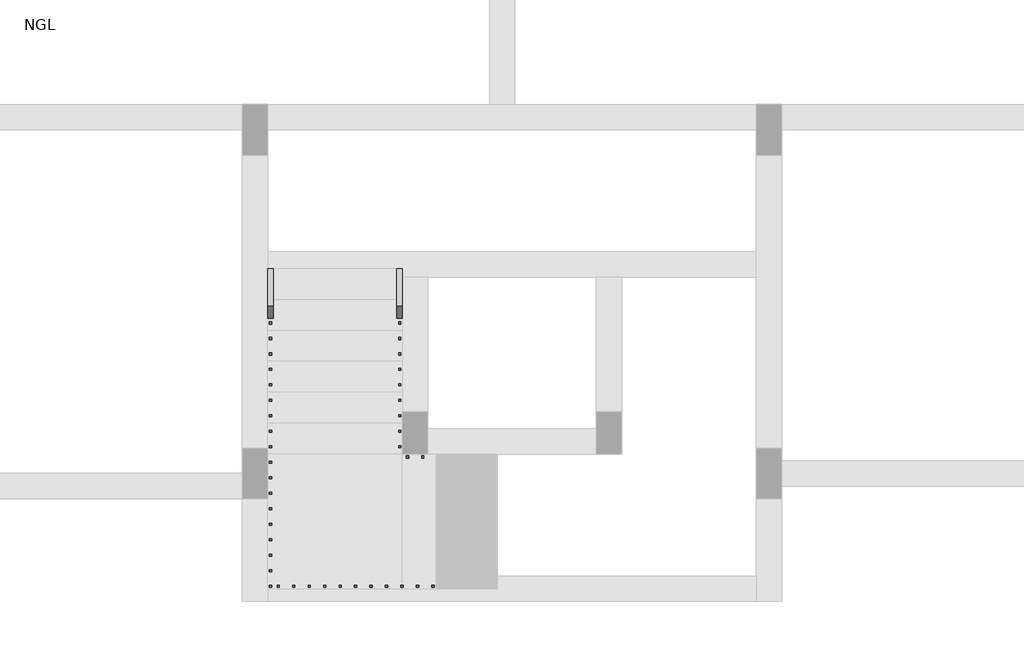
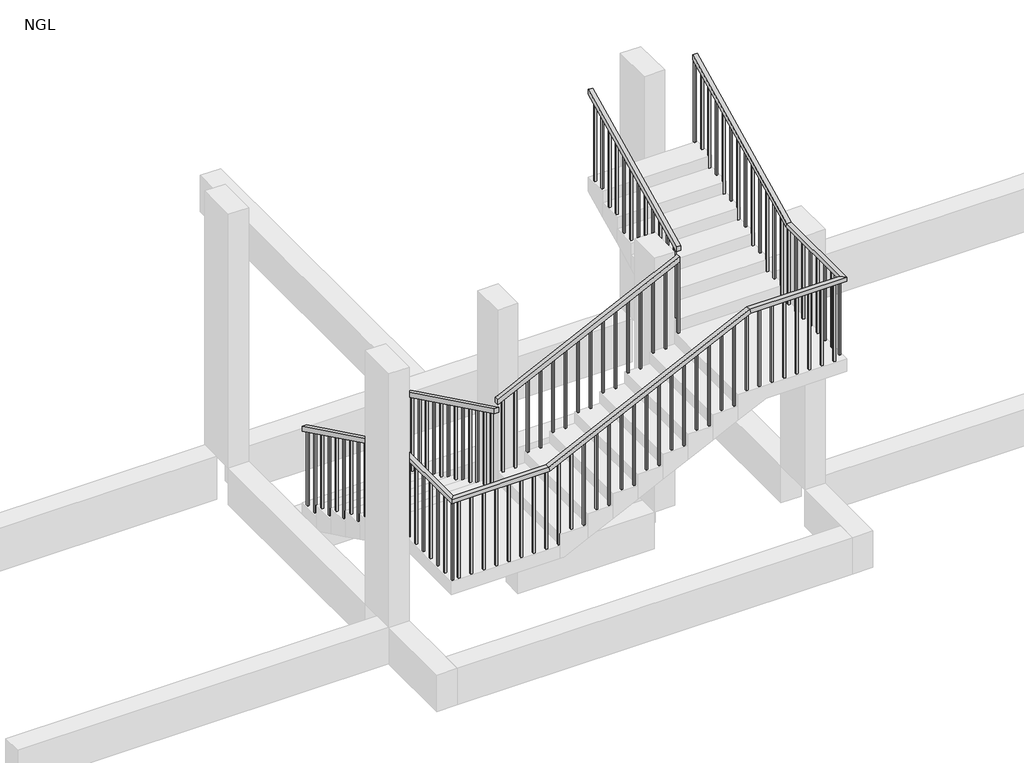
# One storey, part 2 of 2: 2 railings.
"""IFC4 building model written with IfcOpenShell, lengths in millimetres."""

from ifc_helpers import new_model, si_unit, frame, origin, place, context, project, spatial, polyline, outline, extrude, faceted_brep, element, save

model = new_model("IFC4")

# Units and contexts
model_context = context("Model", 3, world=origin())
ifc_project = project(units=[si_unit("LENGTHUNIT", "METRE", prefix="MILLI")], contexts=[model_context])

# Site, building, storey
site = spatial("IfcSite", under=ifc_project)
building = spatial("IfcBuilding", under=site)
storey = spatial("IfcBuildingStorey", under=building, Name="NGL", Elevation=0.0)

# Railings
placement = place(None, origin())
element("IfcRailing", 1, ObjectType="900mm", at=placement, inside=storey, context=model_context, shape_type="SolidModel", body=[
    faceted_brep([(5667245.0165246, -3595922.4258983, 1036.3636364), (5667245.0165246, -3595922.4258983, 980.7263867), (5667195.0165246, -3595922.4258983, 980.7263867), (5667195.0165246, -3595922.4258983, 1036.3636364), (5667245.0165246, -3597746.1784624, 1926.4621742), (5667245.0165246, -3597757.7288111, 1876.4621742), (5667195.0165246, -3597757.7288111, 1876.4621742), (5667195.0165246, -3597746.1784624, 1926.4621742), (5667245.0165246, -3598767.6258983, 1876.4621742), (5667245.0165246, -3598767.6258983, 1926.4621742), (5668280.0541869, -3598767.6258983, 1926.4621742), (5668291.4712079, -3598767.6258983, 1876.4621742), (5667195.0165246, -3598817.6258983, 1876.4621742), (5668291.4712079, -3598817.6258983, 1876.4621742), (5667195.0165246, -3598817.6258983, 1926.4621742), (5668280.0541869, -3598817.6258983, 1926.4621742), (5671563.8165246, -3598767.6258983, 2959.9014622), (5671563.8165246, -3598767.6258983, 3009.9014622), (5671563.8165246, -3597746.1784624, 3009.9014622), (5671563.8165246, -3597734.6281137, 2959.9014622), (5671613.8165246, -3598817.6258983, 2959.9014622), (5671613.8165246, -3597734.6281137, 2959.9014622), (5671613.8165246, -3598817.6258983, 3009.9014622), (5671613.8165246, -3597746.1784624, 3009.9014622), (5670528.7788622, -3598767.6258983, 3009.9014622), (5670540.1958832, -3598767.6258983, 2959.9014622), (5670540.1958832, -3598817.6258983, 2959.9014622), (5670528.7788622, -3598817.6258983, 3009.9014622), (5671563.8165246, -3595922.4258983, 3900.0), (5671613.8165246, -3595922.4258983, 3900.0), (5671613.8165246, -3595922.4258983, 3844.3627504), (5671563.8165246, -3595922.4258983, 3844.3627504)], [[[0, 1, 2, 3]], [[1, 0, 4, 5]], [[2, 1, 5, 6]], [[3, 2, 6, 7]], [[0, 3, 7, 4]], [[8, 9, 10, 11]], [[12, 8, 11, 13]], [[14, 12, 13, 15]], [[9, 14, 15, 10]], [[16, 17, 18, 19]], [[20, 16, 19, 21]], [[22, 20, 21, 23]], [[17, 22, 23, 18]], [[5, 4, 9, 8]], [[6, 5, 8, 12]], [[7, 6, 12, 14]], [[4, 7, 14, 9]], [[11, 10, 24, 25]], [[13, 11, 25, 26]], [[15, 13, 26, 27]], [[10, 15, 27, 24]], [[25, 24, 17, 16]], [[26, 25, 16, 20]], [[27, 26, 20, 22]], [[24, 27, 22, 17]], [[28, 29, 30, 31]], [[19, 18, 28, 31]], [[21, 19, 31, 30]], [[23, 21, 30, 29]], [[18, 23, 29, 28]]]),
    extrude(outline(polyline([(-3595932.6258983, 2863.6363636), (-3595932.6258983, 3839.3845503), (-3595912.6258983, 3849.1457269), (-3595912.6258983, 2863.6363636), (-3595932.6258983, 2863.6363636)])), frame((5671578.8165246, 0.0, 0.0), z_axis=(1.0, 0.0, 0.0), x_axis=(0.0, 1.0, 0.0)), (0.0, 0.0, 1.0), 20.0),
    extrude(outline(polyline([(-3596072.6258983, 2863.6363636), (-3596072.6258983, 3771.0563145), (-3596052.6258983, 3780.817491), (-3596052.6258983, 2863.6363636), (-3596072.6258983, 2863.6363636)])), frame((5671578.8165246, 0.0, 0.0), z_axis=(1.0, 0.0, 0.0), x_axis=(0.0, 1.0, 0.0)), (0.0, 0.0, 1.0), 20.0),
    extrude(outline(polyline([(-3596212.6258983, 2727.2727273), (-3596212.6258983, 3702.7280787), (-3596192.6258983, 3712.4892552), (-3596192.6258983, 2727.2727273), (-3596212.6258983, 2727.2727273)])), frame((5671578.8165246, 0.0, 0.0), z_axis=(1.0, 0.0, 0.0), x_axis=(0.0, 1.0, 0.0)), (0.0, 0.0, 1.0), 20.0),
    extrude(outline(polyline([(-3596352.6258983, 2727.2727273), (-3596352.6258983, 3634.3998428), (-3596332.6258983, 3644.1610194), (-3596332.6258983, 2727.2727273), (-3596352.6258983, 2727.2727273)])), frame((5671578.8165246, 0.0, 0.0), z_axis=(1.0, 0.0, 0.0), x_axis=(0.0, 1.0, 0.0)), (0.0, 0.0, 1.0), 20.0),
    extrude(outline(polyline([(-3596492.6258983, 2590.9090909), (-3596492.6258983, 3566.071607), (-3596472.6258983, 3575.8327835), (-3596472.6258983, 2590.9090909), (-3596492.6258983, 2590.9090909)])), frame((5671578.8165246, 0.0, 0.0), z_axis=(1.0, 0.0, 0.0), x_axis=(0.0, 1.0, 0.0)), (0.0, 0.0, 1.0), 20.0),
    extrude(outline(polyline([(-3596632.6258983, 2590.9090909), (-3596632.6258983, 3497.7433712), (-3596612.6258983, 3507.5045477), (-3596612.6258983, 2590.9090909), (-3596632.6258983, 2590.9090909)])), frame((5671578.8165246, 0.0, 0.0), z_axis=(1.0, 0.0, 0.0), x_axis=(0.0, 1.0, 0.0)), (0.0, 0.0, 1.0), 20.0),
    extrude(outline(polyline([(-3596772.6258983, 2454.5454545), (-3596772.6258983, 3429.4151353), (-3596752.6258983, 3439.1763119), (-3596752.6258983, 2454.5454545), (-3596772.6258983, 2454.5454545)])), frame((5671578.8165246, 0.0, 0.0), z_axis=(1.0, 0.0, 0.0), x_axis=(0.0, 1.0, 0.0)), (0.0, 0.0, 1.0), 20.0),
    extrude(outline(polyline([(-3596912.6258983, 2454.5454545), (-3596912.6258983, 3361.0868995), (-3596892.6258983, 3370.8480761), (-3596892.6258983, 2454.5454545), (-3596912.6258983, 2454.5454545)])), frame((5671578.8165246, 0.0, 0.0), z_axis=(1.0, 0.0, 0.0), x_axis=(0.0, 1.0, 0.0)), (0.0, 0.0, 1.0), 20.0),
    extrude(outline(polyline([(-3597052.6258983, 2318.1818182), (-3597052.6258983, 3292.7586637), (-3597032.6258983, 3302.5198402), (-3597032.6258983, 2318.1818182), (-3597052.6258983, 2318.1818182)])), frame((5671578.8165246, 0.0, 0.0), z_axis=(1.0, 0.0, 0.0), x_axis=(0.0, 1.0, 0.0)), (0.0, 0.0, 1.0), 20.0),
    extrude(outline(polyline([(-3597192.6258983, 2318.1818182), (-3597192.6258983, 3224.4304279), (-3597172.6258983, 3234.1916044), (-3597172.6258983, 2318.1818182), (-3597192.6258983, 2318.1818182)])), frame((5671578.8165246, 0.0, 0.0), z_axis=(1.0, 0.0, 0.0), x_axis=(0.0, 1.0, 0.0)), (0.0, 0.0, 1.0), 20.0),
    extrude(outline(polyline([(-3597332.6258983, 2181.8181818), (-3597332.6258983, 3156.0322155), (-3597312.6258983, 3165.6682488), (-3597312.6258983, 2181.8181818), (-3597332.6258983, 2181.8181818)])), frame((5671578.8165246, 0.0, 0.0), z_axis=(1.0, 0.0, 0.0), x_axis=(0.0, 1.0, 0.0)), (0.0, 0.0, 1.0), 20.0),
    extrude(outline(polyline([(-3597472.6258983, 2181.8181818), (-3597472.6258983, 3087.7739562), (-3597452.6258983, 3097.5351327), (-3597452.6258983, 2181.8181818), (-3597472.6258983, 2181.8181818)])), frame((5671578.8165246, 0.0, 0.0), z_axis=(1.0, 0.0, 0.0), x_axis=(0.0, 1.0, 0.0)), (0.0, 0.0, 1.0), 20.0),
    extrude(outline(polyline([(-3597612.6258983, 2045.4545455), (-3597612.6258983, 3019.4457204), (-3597592.6258983, 3029.2068969), (-3597592.6258983, 2045.4545455), (-3597612.6258983, 2045.4545455)])), frame((5671578.8165246, 0.0, 0.0), z_axis=(1.0, 0.0, 0.0), x_axis=(0.0, 1.0, 0.0)), (0.0, 0.0, 1.0), 20.0),
    extrude(outline(polyline([(-3597752.6258983, 2045.4545455), (-3597752.6258983, 2951.1174845), (-3597732.6258983, 2960.8786611), (-3597732.6258983, 2045.4545455), (-3597752.6258983, 2045.4545455)])), frame((5671578.8165246, 0.0, 0.0), z_axis=(1.0, 0.0, 0.0), x_axis=(0.0, 1.0, 0.0)), (0.0, 0.0, 1.0), 20.0),
    extrude(outline(polyline([(5671598.8165246, -3597892.6258983), (5671578.8165246, -3597892.6258983), (5671578.8165246, -3597872.6258983), (5671598.8165246, -3597872.6258983), (5671598.8165246, -3597892.6258983)])), frame((0.0, 0.0, 2045.4545455), z_axis=(0.0, 0.0, 1.0), x_axis=(1.0, 0.0, 0.0)), (0.0, 0.0, 1.0), 914.4469167),
    extrude(outline(polyline([(5671598.8165246, -3598032.6258983), (5671578.8165246, -3598032.6258983), (5671578.8165246, -3598012.6258983), (5671598.8165246, -3598012.6258983), (5671598.8165246, -3598032.6258983)])), frame((0.0, 0.0, 2045.4545455), z_axis=(0.0, 0.0, 1.0), x_axis=(1.0, 0.0, 0.0)), (0.0, 0.0, 1.0), 914.4469167),
    extrude(outline(polyline([(5671598.8165246, -3598172.6258983), (5671578.8165246, -3598172.6258983), (5671578.8165246, -3598152.6258983), (5671598.8165246, -3598152.6258983), (5671598.8165246, -3598172.6258983)])), frame((0.0, 0.0, 2045.4545455), z_axis=(0.0, 0.0, 1.0), x_axis=(1.0, 0.0, 0.0)), (0.0, 0.0, 1.0), 914.4469167),
    extrude(outline(polyline([(5671598.8165246, -3598312.6258983), (5671578.8165246, -3598312.6258983), (5671578.8165246, -3598292.6258983), (5671598.8165246, -3598292.6258983), (5671598.8165246, -3598312.6258983)])), frame((0.0, 0.0, 2045.4545455), z_axis=(0.0, 0.0, 1.0), x_axis=(1.0, 0.0, 0.0)), (0.0, 0.0, 1.0), 914.4469167),
    extrude(outline(polyline([(5671598.8165246, -3598452.6258983), (5671578.8165246, -3598452.6258983), (5671578.8165246, -3598432.6258983), (5671598.8165246, -3598432.6258983), (5671598.8165246, -3598452.6258983)])), frame((0.0, 0.0, 2045.4545455), z_axis=(0.0, 0.0, 1.0), x_axis=(1.0, 0.0, 0.0)), (0.0, 0.0, 1.0), 914.4469167),
    extrude(outline(polyline([(5671598.8165246, -3598592.6258983), (5671578.8165246, -3598592.6258983), (5671578.8165246, -3598572.6258983), (5671598.8165246, -3598572.6258983), (5671598.8165246, -3598592.6258983)])), frame((0.0, 0.0, 2045.4545455), z_axis=(0.0, 0.0, 1.0), x_axis=(1.0, 0.0, 0.0)), (0.0, 0.0, 1.0), 914.4469167),
    extrude(outline(polyline([(5671598.8165246, -3598732.6258983), (5671578.8165246, -3598732.6258983), (5671578.8165246, -3598712.6258983), (5671598.8165246, -3598712.6258983), (5671598.8165246, -3598732.6258983)])), frame((0.0, 0.0, 2045.4545455), z_axis=(0.0, 0.0, 1.0), x_axis=(1.0, 0.0, 0.0)), (0.0, 0.0, 1.0), 914.4469167),
    extrude(outline(polyline([(5671480.0165246, -3598802.6258983), (5671480.0165246, -3598782.6258983), (5671500.0165246, -3598782.6258983), (5671500.0165246, -3598802.6258983), (5671480.0165246, -3598802.6258983)])), frame((0.0, 0.0, 2045.4545455), z_axis=(0.0, 0.0, 1.0), x_axis=(1.0, 0.0, 0.0)), (0.0, 0.0, 1.0), 914.4469167),
    extrude(outline(polyline([(5671340.0165246, -3598802.6258983), (5671340.0165246, -3598782.6258983), (5671360.0165246, -3598782.6258983), (5671360.0165246, -3598802.6258983), (5671340.0165246, -3598802.6258983)])), frame((0.0, 0.0, 2045.4545455), z_axis=(0.0, 0.0, 1.0), x_axis=(1.0, 0.0, 0.0)), (0.0, 0.0, 1.0), 914.4469167),
    extrude(outline(polyline([(5671200.0165246, -3598802.6258983), (5671200.0165246, -3598782.6258983), (5671220.0165246, -3598782.6258983), (5671220.0165246, -3598802.6258983), (5671200.0165246, -3598802.6258983)])), frame((0.0, 0.0, 2045.4545455), z_axis=(0.0, 0.0, 1.0), x_axis=(1.0, 0.0, 0.0)), (0.0, 0.0, 1.0), 914.4469167),
    extrude(outline(polyline([(5671060.0165246, -3598802.6258983), (5671060.0165246, -3598782.6258983), (5671080.0165246, -3598782.6258983), (5671080.0165246, -3598802.6258983), (5671060.0165246, -3598802.6258983)])), frame((0.0, 0.0, 2045.4545455), z_axis=(0.0, 0.0, 1.0), x_axis=(1.0, 0.0, 0.0)), (0.0, 0.0, 1.0), 914.4469167),
    extrude(outline(polyline([(5670920.0165246, -3598802.6258983), (5670920.0165246, -3598782.6258983), (5670940.0165246, -3598782.6258983), (5670940.0165246, -3598802.6258983), (5670920.0165246, -3598802.6258983)])), frame((0.0, 0.0, 2045.4545455), z_axis=(0.0, 0.0, 1.0), x_axis=(1.0, 0.0, 0.0)), (0.0, 0.0, 1.0), 914.4469167),
    extrude(outline(polyline([(5670780.0165246, -3598802.6258983), (5670780.0165246, -3598782.6258983), (5670800.0165246, -3598782.6258983), (5670800.0165246, -3598802.6258983), (5670780.0165246, -3598802.6258983)])), frame((0.0, 0.0, 2045.4545455), z_axis=(0.0, 0.0, 1.0), x_axis=(1.0, 0.0, 0.0)), (0.0, 0.0, 1.0), 914.4469167),
    extrude(outline(polyline([(5670640.0165246, -3598802.6258983), (5670640.0165246, -3598782.6258983), (5670660.0165246, -3598782.6258983), (5670660.0165246, -3598802.6258983), (5670640.0165246, -3598802.6258983)])), frame((0.0, 0.0, 2045.4545455), z_axis=(0.0, 0.0, 1.0), x_axis=(1.0, 0.0, 0.0)), (0.0, 0.0, 1.0), 914.4469167),
    extrude(outline(polyline([(2940.5429804, 5670500.0165246), (2045.4545455, 5670500.0165246), (2045.4545455, 5670520.0165246), (2950.1790136, 5670520.0165246), (2940.5429804, 5670500.0165246)])), frame((0.0, -3598802.6258983, 0.0), z_axis=(0.0, 1.0, 0.0), x_axis=(0.0, 0.0, 1.0)), (0.0, 0.0, 1.0), 20.0),
    extrude(outline(polyline([(2873.0907476, 5670360.0165246), (1909.0909091, 5670360.0165246), (1909.0909091, 5670380.0165246), (2882.7267808, 5670380.0165246), (2873.0907476, 5670360.0165246)])), frame((0.0, -3598802.6258983, 0.0), z_axis=(0.0, 1.0, 0.0), x_axis=(0.0, 0.0, 1.0)), (0.0, 0.0, 1.0), 20.0),
    extrude(outline(polyline([(2805.6385148, 5670220.0165246), (1909.0909091, 5670220.0165246), (1909.0909091, 5670240.0165246), (2815.274548, 5670240.0165246), (2805.6385148, 5670220.0165246)])), frame((0.0, -3598802.6258983, 0.0), z_axis=(0.0, 1.0, 0.0), x_axis=(0.0, 0.0, 1.0)), (0.0, 0.0, 1.0), 20.0),
    extrude(outline(polyline([(2738.186282, 5670080.0165246), (1772.7272727, 5670080.0165246), (1772.7272727, 5670100.0165246), (2747.8223152, 5670100.0165246), (2738.186282, 5670080.0165246)])), frame((0.0, -3598802.6258983, 0.0), z_axis=(0.0, 1.0, 0.0), x_axis=(0.0, 0.0, 1.0)), (0.0, 0.0, 1.0), 20.0),
    extrude(outline(polyline([(2670.7340492, 5669940.0165246), (1772.7272727, 5669940.0165246), (1772.7272727, 5669960.0165246), (2680.3700824, 5669960.0165246), (2670.7340492, 5669940.0165246)])), frame((0.0, -3598802.6258983, 0.0), z_axis=(0.0, 1.0, 0.0), x_axis=(0.0, 0.0, 1.0)), (0.0, 0.0, 1.0), 20.0),
    extrude(outline(polyline([(2603.2818163, 5669800.0165246), (1636.3636364, 5669800.0165246), (1636.3636364, 5669820.0165246), (2612.9178496, 5669820.0165246), (2603.2818163, 5669800.0165246)])), frame((0.0, -3598802.6258983, 0.0), z_axis=(0.0, 1.0, 0.0), x_axis=(0.0, 0.0, 1.0)), (0.0, 0.0, 1.0), 20.0),
    extrude(outline(polyline([(2535.8295835, 5669660.0165246), (1636.3636364, 5669660.0165246), (1636.3636364, 5669680.0165246), (2545.4656168, 5669680.0165246), (2535.8295835, 5669660.0165246)])), frame((0.0, -3598802.6258983, 0.0), z_axis=(0.0, 1.0, 0.0), x_axis=(0.0, 0.0, 1.0)), (0.0, 0.0, 1.0), 20.0),
    extrude(outline(polyline([(2468.3773507, 5669520.0165246), (1500.0, 5669520.0165246), (1500.0, 5669540.0165246), (2478.013384, 5669540.0165246), (2468.3773507, 5669520.0165246)])), frame((0.0, -3598802.6258983, 0.0), z_axis=(0.0, 1.0, 0.0), x_axis=(0.0, 0.0, 1.0)), (0.0, 0.0, 1.0), 20.0),
    extrude(outline(polyline([(2400.9251179, 5669380.0165246), (1500.0, 5669380.0165246), (1500.0, 5669400.0165246), (2410.5611512, 5669400.0165246), (2400.9251179, 5669380.0165246)])), frame((0.0, -3598802.6258983, 0.0), z_axis=(0.0, 1.0, 0.0), x_axis=(0.0, 0.0, 1.0)), (0.0, 0.0, 1.0), 20.0),
    extrude(outline(polyline([(2333.4728851, 5669240.0165246), (1363.6363636, 5669240.0165246), (1363.6363636, 5669260.0165246), (2343.1089184, 5669260.0165246), (2333.4728851, 5669240.0165246)])), frame((0.0, -3598802.6258983, 0.0), z_axis=(0.0, 1.0, 0.0), x_axis=(0.0, 0.0, 1.0)), (0.0, 0.0, 1.0), 20.0),
    extrude(outline(polyline([(2266.0206523, 5669100.0165246), (1363.6363636, 5669100.0165246), (1363.6363636, 5669120.0165246), (2275.6566856, 5669120.0165246), (2266.0206523, 5669100.0165246)])), frame((0.0, -3598802.6258983, 0.0), z_axis=(0.0, 1.0, 0.0), x_axis=(0.0, 0.0, 1.0)), (0.0, 0.0, 1.0), 20.0),
    extrude(outline(polyline([(2198.5684195, 5668960.0165246), (1227.2727273, 5668960.0165246), (1227.2727273, 5668980.0165246), (2208.2044528, 5668980.0165246), (2198.5684195, 5668960.0165246)])), frame((0.0, -3598802.6258983, 0.0), z_axis=(0.0, 1.0, 0.0), x_axis=(0.0, 0.0, 1.0)), (0.0, 0.0, 1.0), 20.0),
    extrude(outline(polyline([(2131.1161867, 5668820.0165246), (1227.2727273, 5668820.0165246), (1227.2727273, 5668840.0165246), (2140.75222, 5668840.0165246), (2131.1161867, 5668820.0165246)])), frame((0.0, -3598802.6258983, 0.0), z_axis=(0.0, 1.0, 0.0), x_axis=(0.0, 0.0, 1.0)), (0.0, 0.0, 1.0), 20.0),
    extrude(outline(polyline([(2063.6639539, 5668680.0165246), (1090.9090909, 5668680.0165246), (1090.9090909, 5668700.0165246), (2073.2999871, 5668700.0165246), (2063.6639539, 5668680.0165246)])), frame((0.0, -3598802.6258983, 0.0), z_axis=(0.0, 1.0, 0.0), x_axis=(0.0, 0.0, 1.0)), (0.0, 0.0, 1.0), 20.0),
    extrude(outline(polyline([(1996.2117211, 5668540.0165246), (1090.9090909, 5668540.0165246), (1090.9090909, 5668560.0165246), (2005.8477543, 5668560.0165246), (1996.2117211, 5668540.0165246)])), frame((0.0, -3598802.6258983, 0.0), z_axis=(0.0, 1.0, 0.0), x_axis=(0.0, 0.0, 1.0)), (0.0, 0.0, 1.0), 20.0),
    extrude(outline(polyline([(1928.7594883, 5668400.0165246), (954.5454545, 5668400.0165246), (954.5454545, 5668420.0165246), (1938.3955215, 5668420.0165246), (1928.7594883, 5668400.0165246)])), frame((0.0, -3598802.6258983, 0.0), z_axis=(0.0, 1.0, 0.0), x_axis=(0.0, 0.0, 1.0)), (0.0, 0.0, 1.0), 20.0),
    extrude(outline(polyline([(5668260.0165246, -3598802.6258983), (5668260.0165246, -3598782.6258983), (5668280.0165246, -3598782.6258983), (5668280.0165246, -3598802.6258983), (5668260.0165246, -3598802.6258983)])), frame((0.0, 0.0, 954.5454545), z_axis=(0.0, 0.0, 1.0), x_axis=(1.0, 0.0, 0.0)), (0.0, 0.0, 1.0), 921.9167196),
    extrude(outline(polyline([(5668120.0165246, -3598802.6258983), (5668120.0165246, -3598782.6258983), (5668140.0165246, -3598782.6258983), (5668140.0165246, -3598802.6258983), (5668120.0165246, -3598802.6258983)])), frame((0.0, 0.0, 954.5454545), z_axis=(0.0, 0.0, 1.0), x_axis=(1.0, 0.0, 0.0)), (0.0, 0.0, 1.0), 921.9167196),
    extrude(outline(polyline([(5667980.0165246, -3598802.6258983), (5667980.0165246, -3598782.6258983), (5668000.0165246, -3598782.6258983), (5668000.0165246, -3598802.6258983), (5667980.0165246, -3598802.6258983)])), frame((0.0, 0.0, 954.5454545), z_axis=(0.0, 0.0, 1.0), x_axis=(1.0, 0.0, 0.0)), (0.0, 0.0, 1.0), 921.9167196),
    extrude(outline(polyline([(5667840.0165246, -3598802.6258983), (5667840.0165246, -3598782.6258983), (5667860.0165246, -3598782.6258983), (5667860.0165246, -3598802.6258983), (5667840.0165246, -3598802.6258983)])), frame((0.0, 0.0, 954.5454545), z_axis=(0.0, 0.0, 1.0), x_axis=(1.0, 0.0, 0.0)), (0.0, 0.0, 1.0), 921.9167196),
    extrude(outline(polyline([(5667700.0165246, -3598802.6258983), (5667700.0165246, -3598782.6258983), (5667720.0165246, -3598782.6258983), (5667720.0165246, -3598802.6258983), (5667700.0165246, -3598802.6258983)])), frame((0.0, 0.0, 954.5454545), z_axis=(0.0, 0.0, 1.0), x_axis=(1.0, 0.0, 0.0)), (0.0, 0.0, 1.0), 921.9167196),
    extrude(outline(polyline([(5667560.0165246, -3598802.6258983), (5667560.0165246, -3598782.6258983), (5667580.0165246, -3598782.6258983), (5667580.0165246, -3598802.6258983), (5667560.0165246, -3598802.6258983)])), frame((0.0, 0.0, 954.5454545), z_axis=(0.0, 0.0, 1.0), x_axis=(1.0, 0.0, 0.0)), (0.0, 0.0, 1.0), 921.9167196),
    extrude(outline(polyline([(5667420.0165246, -3598802.6258983), (5667420.0165246, -3598782.6258983), (5667440.0165246, -3598782.6258983), (5667440.0165246, -3598802.6258983), (5667420.0165246, -3598802.6258983)])), frame((0.0, 0.0, 954.5454545), z_axis=(0.0, 0.0, 1.0), x_axis=(1.0, 0.0, 0.0)), (0.0, 0.0, 1.0), 921.9167196),
    extrude(outline(polyline([(5667280.0165246, -3598802.6258983), (5667280.0165246, -3598782.6258983), (5667300.0165246, -3598782.6258983), (5667300.0165246, -3598802.6258983), (5667280.0165246, -3598802.6258983)])), frame((0.0, 0.0, 954.5454545), z_axis=(0.0, 0.0, 1.0), x_axis=(1.0, 0.0, 0.0)), (0.0, 0.0, 1.0), 921.9167196),
    extrude(outline(polyline([(5667210.0165246, -3598782.4258983), (5667230.0165246, -3598782.4258983), (5667230.0165246, -3598802.4258983), (5667210.0165246, -3598802.4258983), (5667210.0165246, -3598782.4258983)])), frame((0.0, 0.0, 954.5454545), z_axis=(0.0, 0.0, 1.0), x_axis=(1.0, 0.0, 0.0)), (0.0, 0.0, 1.0), 921.9167196),
    extrude(outline(polyline([(5667210.0165246, -3598642.4258983), (5667230.0165246, -3598642.4258983), (5667230.0165246, -3598662.4258983), (5667210.0165246, -3598662.4258983), (5667210.0165246, -3598642.4258983)])), frame((0.0, 0.0, 954.5454545), z_axis=(0.0, 0.0, 1.0), x_axis=(1.0, 0.0, 0.0)), (0.0, 0.0, 1.0), 921.9167196),
    extrude(outline(polyline([(5667210.0165246, -3598502.4258983), (5667230.0165246, -3598502.4258983), (5667230.0165246, -3598522.4258983), (5667210.0165246, -3598522.4258983), (5667210.0165246, -3598502.4258983)])), frame((0.0, 0.0, 954.5454545), z_axis=(0.0, 0.0, 1.0), x_axis=(1.0, 0.0, 0.0)), (0.0, 0.0, 1.0), 921.9167196),
    extrude(outline(polyline([(5667210.0165246, -3598362.4258983), (5667230.0165246, -3598362.4258983), (5667230.0165246, -3598382.4258983), (5667210.0165246, -3598382.4258983), (5667210.0165246, -3598362.4258983)])), frame((0.0, 0.0, 954.5454545), z_axis=(0.0, 0.0, 1.0), x_axis=(1.0, 0.0, 0.0)), (0.0, 0.0, 1.0), 921.9167196),
    extrude(outline(polyline([(5667210.0165246, -3598222.4258983), (5667230.0165246, -3598222.4258983), (5667230.0165246, -3598242.4258983), (5667210.0165246, -3598242.4258983), (5667210.0165246, -3598222.4258983)])), frame((0.0, 0.0, 954.5454545), z_axis=(0.0, 0.0, 1.0), x_axis=(1.0, 0.0, 0.0)), (0.0, 0.0, 1.0), 921.9167196),
    extrude(outline(polyline([(5667210.0165246, -3598082.4258983), (5667230.0165246, -3598082.4258983), (5667230.0165246, -3598102.4258983), (5667210.0165246, -3598102.4258983), (5667210.0165246, -3598082.4258983)])), frame((0.0, 0.0, 954.5454545), z_axis=(0.0, 0.0, 1.0), x_axis=(1.0, 0.0, 0.0)), (0.0, 0.0, 1.0), 921.9167196),
    extrude(outline(polyline([(5667210.0165246, -3597942.4258983), (5667230.0165246, -3597942.4258983), (5667230.0165246, -3597962.4258983), (5667210.0165246, -3597962.4258983), (5667210.0165246, -3597942.4258983)])), frame((0.0, 0.0, 954.5454545), z_axis=(0.0, 0.0, 1.0), x_axis=(1.0, 0.0, 0.0)), (0.0, 0.0, 1.0), 921.9167196),
    extrude(outline(polyline([(5667210.0165246, -3597802.4258983), (5667230.0165246, -3597802.4258983), (5667230.0165246, -3597822.4258983), (5667210.0165246, -3597822.4258983), (5667210.0165246, -3597802.4258983)])), frame((0.0, 0.0, 954.5454545), z_axis=(0.0, 0.0, 1.0), x_axis=(1.0, 0.0, 0.0)), (0.0, 0.0, 1.0), 921.9167196),
    extrude(outline(polyline([(-3597662.4258983, 1829.9487463), (-3597662.4258983, 954.5454545), (-3597682.4258983, 954.5454545), (-3597682.4258983, 1839.7099229), (-3597662.4258983, 1829.9487463)])), frame((5667210.0165246, 0.0, 0.0), z_axis=(1.0, 0.0, 0.0), x_axis=(0.0, 1.0, 0.0)), (0.0, 0.0, 1.0), 20.0),
    extrude(outline(polyline([(-3597522.4258983, 1761.6205105), (-3597522.4258983, 818.1818182), (-3597542.4258983, 818.1818182), (-3597542.4258983, 1771.381687), (-3597522.4258983, 1761.6205105)])), frame((5667210.0165246, 0.0, 0.0), z_axis=(1.0, 0.0, 0.0), x_axis=(0.0, 1.0, 0.0)), (0.0, 0.0, 1.0), 20.0),
    extrude(outline(polyline([(-3597382.4258983, 1693.2922747), (-3597382.4258983, 818.1818182), (-3597402.4258983, 818.1818182), (-3597402.4258983, 1703.0534512), (-3597382.4258983, 1693.2922747)])), frame((5667210.0165246, 0.0, 0.0), z_axis=(1.0, 0.0, 0.0), x_axis=(0.0, 1.0, 0.0)), (0.0, 0.0, 1.0), 20.0),
    extrude(outline(polyline([(-3597242.4258983, 1624.9640388), (-3597242.4258983, 681.8181818), (-3597262.4258983, 681.8181818), (-3597262.4258983, 1634.7252154), (-3597242.4258983, 1624.9640388)])), frame((5667210.0165246, 0.0, 0.0), z_axis=(1.0, 0.0, 0.0), x_axis=(0.0, 1.0, 0.0)), (0.0, 0.0, 1.0), 20.0),
    extrude(outline(polyline([(-3597102.4258983, 1556.635803), (-3597102.4258983, 681.8181818), (-3597122.4258983, 681.8181818), (-3597122.4258983, 1566.3969796), (-3597102.4258983, 1556.635803)])), frame((5667210.0165246, 0.0, 0.0), z_axis=(1.0, 0.0, 0.0), x_axis=(0.0, 1.0, 0.0)), (0.0, 0.0, 1.0), 20.0),
    extrude(outline(polyline([(-3596962.4258983, 1488.3075672), (-3596962.4258983, 545.4545455), (-3596982.4258983, 545.4545455), (-3596982.4258983, 1498.0687437), (-3596962.4258983, 1488.3075672)])), frame((5667210.0165246, 0.0, 0.0), z_axis=(1.0, 0.0, 0.0), x_axis=(0.0, 1.0, 0.0)), (0.0, 0.0, 1.0), 20.0),
    extrude(outline(polyline([(-3596822.4258983, 1419.9793313), (-3596822.4258983, 545.4545455), (-3596842.4258983, 545.4545455), (-3596842.4258983, 1429.7405079), (-3596822.4258983, 1419.9793313)])), frame((5667210.0165246, 0.0, 0.0), z_axis=(1.0, 0.0, 0.0), x_axis=(0.0, 1.0, 0.0)), (0.0, 0.0, 1.0), 20.0),
    extrude(outline(polyline([(-3596682.4258983, 1351.6510955), (-3596682.4258983, 409.0909091), (-3596702.4258983, 409.0909091), (-3596702.4258983, 1361.4122721), (-3596682.4258983, 1351.6510955)])), frame((5667210.0165246, 0.0, 0.0), z_axis=(1.0, 0.0, 0.0), x_axis=(0.0, 1.0, 0.0)), (0.0, 0.0, 1.0), 20.0),
    extrude(outline(polyline([(-3596542.4258983, 1283.3228597), (-3596542.4258983, 409.0909091), (-3596562.4258983, 409.0909091), (-3596562.4258983, 1293.0840362), (-3596542.4258983, 1283.3228597)])), frame((5667210.0165246, 0.0, 0.0), z_axis=(1.0, 0.0, 0.0), x_axis=(0.0, 1.0, 0.0)), (0.0, 0.0, 1.0), 20.0),
    extrude(outline(polyline([(-3596402.4258983, 1214.9946239), (-3596402.4258983, 272.7272727), (-3596422.4258983, 272.7272727), (-3596422.4258983, 1224.7558004), (-3596402.4258983, 1214.9946239)])), frame((5667210.0165246, 0.0, 0.0), z_axis=(1.0, 0.0, 0.0), x_axis=(0.0, 1.0, 0.0)), (0.0, 0.0, 1.0), 20.0),
    extrude(outline(polyline([(-3596262.4258983, 1146.666388), (-3596262.4258983, 272.7272727), (-3596282.4258983, 272.7272727), (-3596282.4258983, 1156.4275646), (-3596262.4258983, 1146.666388)])), frame((5667210.0165246, 0.0, 0.0), z_axis=(1.0, 0.0, 0.0), x_axis=(0.0, 1.0, 0.0)), (0.0, 0.0, 1.0), 20.0),
    extrude(outline(polyline([(-3596122.4258983, 1078.3381522), (-3596122.4258983, 136.3636364), (-3596142.4258983, 136.3636364), (-3596142.4258983, 1088.0993287), (-3596122.4258983, 1078.3381522)])), frame((5667210.0165246, 0.0, 0.0), z_axis=(1.0, 0.0, 0.0), x_axis=(0.0, 1.0, 0.0)), (0.0, 0.0, 1.0), 20.0),
    extrude(outline(polyline([(-3595982.4258983, 1010.0099164), (-3595982.4258983, 136.3636364), (-3596002.4258983, 136.3636364), (-3596002.4258983, 1019.7710929), (-3595982.4258983, 1010.0099164)])), frame((5667210.0165246, 0.0, 0.0), z_axis=(1.0, 0.0, 0.0), x_axis=(0.0, 1.0, 0.0)), (0.0, 0.0, 1.0), 20.0),
])
element("IfcRailing", 2, ObjectType="900mm", at=placement, inside=storey, context=model_context, shape_type="SweptSolid", body=[
    extrude(outline(polyline([(-3595922.4258983, 1036.3636364), (-3595922.4258983, 980.7263867), (-3597624.2258983, 1811.3048991), (-3597624.2258983, 1866.9421488), (-3595922.4258983, 1036.3636364)])), frame((5668363.4165246, 0.0, 0.0), z_axis=(1.0, 0.0, 0.0), x_axis=(0.0, 1.0, 0.0)), (0.0, 0.0, 1.0), 50.0),
    extrude(outline(polyline([(1978.6713287, 5668388.4165246), (1923.170589, 5668388.4165246), (2902.191568, 5670420.4165245), (2957.6923077, 5670420.4165245), (1978.6713287, 5668388.4165246)])), frame((0.0, -3597649.2258983, 0.0), z_axis=(0.0, 1.0, 0.0), x_axis=(0.0, 0.0, 1.0)), (0.0, 0.0, 1.0), 50.0),
    extrude(outline(polyline([(-3597624.2258983, 3013.784238), (-3597624.2258983, 3069.4214876), (-3595922.4258983, 3900.0), (-3595922.4258983, 3844.3627504), (-3597624.2258983, 3013.784238)])), frame((5670395.4165245, 0.0, 0.0), z_axis=(1.0, 0.0, 0.0), x_axis=(0.0, 1.0, 0.0)), (0.0, 0.0, 1.0), 50.0),
    extrude(outline(polyline([(-3596024.2258983, 3794.6783617), (-3596004.2258983, 3804.4395383), (-3596004.2258983, 2863.6363636), (-3596024.2258983, 2863.6363636), (-3596024.2258983, 3794.6783617)])), frame((5670410.4165245, 0.0, 0.0), z_axis=(1.0, 0.0, 0.0), x_axis=(0.0, 1.0, 0.0)), (0.0, 0.0, 1.0), 20.0),
    extrude(outline(polyline([(-3596164.2258983, 3726.3501259), (-3596144.2258983, 3736.1113025), (-3596144.2258983, 2863.6363636), (-3596164.2258983, 2863.6363636), (-3596164.2258983, 3726.3501259)])), frame((5670410.4165245, 0.0, 0.0), z_axis=(1.0, 0.0, 0.0), x_axis=(0.0, 1.0, 0.0)), (0.0, 0.0, 1.0), 20.0),
    extrude(outline(polyline([(-3596304.2258983, 3658.0218901), (-3596284.2258983, 3667.7830666), (-3596284.2258983, 2727.2727273), (-3596304.2258983, 2727.2727273), (-3596304.2258983, 3658.0218901)])), frame((5670410.4165245, 0.0, 0.0), z_axis=(1.0, 0.0, 0.0), x_axis=(0.0, 1.0, 0.0)), (0.0, 0.0, 1.0), 20.0),
    extrude(outline(polyline([(-3596444.2258983, 3589.6936542), (-3596424.2258983, 3599.4548308), (-3596424.2258983, 2727.2727273), (-3596444.2258983, 2727.2727273), (-3596444.2258983, 3589.6936542)])), frame((5670410.4165245, 0.0, 0.0), z_axis=(1.0, 0.0, 0.0), x_axis=(0.0, 1.0, 0.0)), (0.0, 0.0, 1.0), 20.0),
    extrude(outline(polyline([(-3596584.2258983, 3521.3654184), (-3596564.2258983, 3531.126595), (-3596564.2258983, 2590.9090909), (-3596584.2258983, 2590.9090909), (-3596584.2258983, 3521.3654184)])), frame((5670410.4165245, 0.0, 0.0), z_axis=(1.0, 0.0, 0.0), x_axis=(0.0, 1.0, 0.0)), (0.0, 0.0, 1.0), 20.0),
    extrude(outline(polyline([(-3596724.2258983, 3453.0371826), (-3596704.2258983, 3462.7983591), (-3596704.2258983, 2590.9090909), (-3596724.2258983, 2590.9090909), (-3596724.2258983, 3453.0371826)])), frame((5670410.4165245, 0.0, 0.0), z_axis=(1.0, 0.0, 0.0), x_axis=(0.0, 1.0, 0.0)), (0.0, 0.0, 1.0), 20.0),
    extrude(outline(polyline([(-3596864.2258983, 3384.7089468), (-3596844.2258983, 3394.4701233), (-3596844.2258983, 2454.5454545), (-3596864.2258983, 2454.5454545), (-3596864.2258983, 3384.7089468)])), frame((5670410.4165245, 0.0, 0.0), z_axis=(1.0, 0.0, 0.0), x_axis=(0.0, 1.0, 0.0)), (0.0, 0.0, 1.0), 20.0),
    extrude(outline(polyline([(-3597004.2258983, 3316.3807109), (-3596984.2258983, 3326.1418875), (-3596984.2258983, 2454.5454545), (-3597004.2258983, 2454.5454545), (-3597004.2258983, 3316.3807109)])), frame((5670410.4165245, 0.0, 0.0), z_axis=(1.0, 0.0, 0.0), x_axis=(0.0, 1.0, 0.0)), (0.0, 0.0, 1.0), 20.0),
    extrude(outline(polyline([(-3597144.2258983, 3248.0524751), (-3597124.2258983, 3257.8136516), (-3597124.2258983, 2318.1818182), (-3597144.2258983, 2318.1818182), (-3597144.2258983, 3248.0524751)])), frame((5670410.4165245, 0.0, 0.0), z_axis=(1.0, 0.0, 0.0), x_axis=(0.0, 1.0, 0.0)), (0.0, 0.0, 1.0), 20.0),
    extrude(outline(polyline([(-3597284.2258983, 3179.7242393), (-3597264.2258983, 3189.4854158), (-3597264.2258983, 2318.1818182), (-3597284.2258983, 2318.1818182), (-3597284.2258983, 3179.7242393)])), frame((5670410.4165245, 0.0, 0.0), z_axis=(1.0, 0.0, 0.0), x_axis=(0.0, 1.0, 0.0)), (0.0, 0.0, 1.0), 20.0),
    extrude(outline(polyline([(-3597424.2258983, 3111.3960034), (-3597404.2258983, 3121.15718), (-3597404.2258983, 2181.8181818), (-3597424.2258983, 2181.8181818), (-3597424.2258983, 3111.3960034)])), frame((5670410.4165245, 0.0, 0.0), z_axis=(1.0, 0.0, 0.0), x_axis=(0.0, 1.0, 0.0)), (0.0, 0.0, 1.0), 20.0),
    extrude(outline(polyline([(-3597564.2258983, 3042.9877797), (-3597544.2258983, 3052.6238129), (-3597544.2258983, 2181.8181818), (-3597564.2258983, 2181.8181818), (-3597564.2258983, 3042.9877797)])), frame((5670410.4165245, 0.0, 0.0), z_axis=(1.0, 0.0, 0.0), x_axis=(0.0, 1.0, 0.0)), (0.0, 0.0, 1.0), 20.0),
    extrude(outline(polyline([(2045.4545455, 5670408.4165246), (2045.4545455, 5670428.4165246), (2906.0459813, 5670428.4165246), (2896.4099481, 5670408.4165246), (2045.4545455, 5670408.4165246)])), frame((0.0, -3597634.2258983, 0.0), z_axis=(0.0, 1.0, 0.0), x_axis=(0.0, 0.0, 1.0)), (0.0, 0.0, 1.0), 20.0),
    extrude(outline(polyline([(1909.0909091, 5670268.4165246), (1909.0909091, 5670288.4165246), (2838.5937485, 5670288.4165246), (2828.9577152, 5670268.4165246), (1909.0909091, 5670268.4165246)])), frame((0.0, -3597634.2258983, 0.0), z_axis=(0.0, 1.0, 0.0), x_axis=(0.0, 0.0, 1.0)), (0.0, 0.0, 1.0), 20.0),
    extrude(outline(polyline([(1909.0909091, 5670128.4165246), (1909.0909091, 5670148.4165246), (2771.1415157, 5670148.4165246), (2761.5054824, 5670128.4165246), (1909.0909091, 5670128.4165246)])), frame((0.0, -3597634.2258983, 0.0), z_axis=(0.0, 1.0, 0.0), x_axis=(0.0, 0.0, 1.0)), (0.0, 0.0, 1.0), 20.0),
    extrude(outline(polyline([(1772.7272727, 5669988.4165246), (1772.7272727, 5670008.4165246), (2703.6892829, 5670008.4165246), (2694.0532496, 5669988.4165246), (1772.7272727, 5669988.4165246)])), frame((0.0, -3597634.2258983, 0.0), z_axis=(0.0, 1.0, 0.0), x_axis=(0.0, 0.0, 1.0)), (0.0, 0.0, 1.0), 20.0),
    extrude(outline(polyline([(1772.7272727, 5669848.4165246), (1772.7272727, 5669868.4165246), (2636.2370501, 5669868.4165246), (2626.6010168, 5669848.4165246), (1772.7272727, 5669848.4165246)])), frame((0.0, -3597634.2258983, 0.0), z_axis=(0.0, 1.0, 0.0), x_axis=(0.0, 0.0, 1.0)), (0.0, 0.0, 1.0), 20.0),
    extrude(outline(polyline([(1636.3636364, 5669708.4165246), (1636.3636364, 5669728.4165246), (2568.7848173, 5669728.4165246), (2559.148784, 5669708.4165246), (1636.3636364, 5669708.4165246)])), frame((0.0, -3597634.2258983, 0.0), z_axis=(0.0, 1.0, 0.0), x_axis=(0.0, 0.0, 1.0)), (0.0, 0.0, 1.0), 20.0),
    extrude(outline(polyline([(1636.3636364, 5669568.4165246), (1636.3636364, 5669588.4165246), (2501.3325845, 5669588.4165246), (2491.6965512, 5669568.4165246), (1636.3636364, 5669568.4165246)])), frame((0.0, -3597634.2258983, 0.0), z_axis=(0.0, 1.0, 0.0), x_axis=(0.0, 0.0, 1.0)), (0.0, 0.0, 1.0), 20.0),
    extrude(outline(polyline([(1500.0, 5669428.4165246), (1500.0, 5669448.4165246), (2433.8803517, 5669448.4165246), (2424.2443184, 5669428.4165246), (1500.0, 5669428.4165246)])), frame((0.0, -3597634.2258983, 0.0), z_axis=(0.0, 1.0, 0.0), x_axis=(0.0, 0.0, 1.0)), (0.0, 0.0, 1.0), 20.0),
    extrude(outline(polyline([(1500.0, 5669288.4165246), (1500.0, 5669308.4165246), (2366.4281189, 5669308.4165246), (2356.7920856, 5669288.4165246), (1500.0, 5669288.4165246)])), frame((0.0, -3597634.2258983, 0.0), z_axis=(0.0, 1.0, 0.0), x_axis=(0.0, 0.0, 1.0)), (0.0, 0.0, 1.0), 20.0),
    extrude(outline(polyline([(1363.6363636, 5669148.4165246), (1363.6363636, 5669168.4165246), (2298.9758861, 5669168.4165246), (2289.3398528, 5669148.4165246), (1363.6363636, 5669148.4165246)])), frame((0.0, -3597634.2258983, 0.0), z_axis=(0.0, 1.0, 0.0), x_axis=(0.0, 0.0, 1.0)), (0.0, 0.0, 1.0), 20.0),
    extrude(outline(polyline([(1363.6363636, 5669008.4165246), (1363.6363636, 5669028.4165246), (2231.5236532, 5669028.4165246), (2221.88762, 5669008.4165246), (1363.6363636, 5669008.4165246)])), frame((0.0, -3597634.2258983, 0.0), z_axis=(0.0, 1.0, 0.0), x_axis=(0.0, 0.0, 1.0)), (0.0, 0.0, 1.0), 20.0),
    extrude(outline(polyline([(1227.2727273, 5668868.4165246), (1227.2727273, 5668888.4165246), (2164.0714204, 5668888.4165246), (2154.4353872, 5668868.4165246), (1227.2727273, 5668868.4165246)])), frame((0.0, -3597634.2258983, 0.0), z_axis=(0.0, 1.0, 0.0), x_axis=(0.0, 0.0, 1.0)), (0.0, 0.0, 1.0), 20.0),
    extrude(outline(polyline([(1227.2727273, 5668728.4165246), (1227.2727273, 5668748.4165246), (2096.6191876, 5668748.4165246), (2086.9831544, 5668728.4165246), (1227.2727273, 5668728.4165246)])), frame((0.0, -3597634.2258983, 0.0), z_axis=(0.0, 1.0, 0.0), x_axis=(0.0, 0.0, 1.0)), (0.0, 0.0, 1.0), 20.0),
    extrude(outline(polyline([(1090.9090909, 5668588.4165246), (1090.9090909, 5668608.4165246), (2029.1669548, 5668608.4165246), (2019.5309216, 5668588.4165246), (1090.9090909, 5668588.4165246)])), frame((0.0, -3597634.2258983, 0.0), z_axis=(0.0, 1.0, 0.0), x_axis=(0.0, 0.0, 1.0)), (0.0, 0.0, 1.0), 20.0),
    extrude(outline(polyline([(1090.9090909, 5668448.4165246), (1090.9090909, 5668468.4165246), (1961.714722, 5668468.4165246), (1952.0786888, 5668448.4165246), (1090.9090909, 5668448.4165246)])), frame((0.0, -3597634.2258983, 0.0), z_axis=(0.0, 1.0, 0.0), x_axis=(0.0, 0.0, 1.0)), (0.0, 0.0, 1.0), 20.0),
    extrude(outline(polyline([(-3597522.4258983, 818.1818182), (-3597542.4258983, 818.1818182), (-3597542.4258983, 1771.381687), (-3597522.4258983, 1761.6205105), (-3597522.4258983, 818.1818182)])), frame((5668378.4165246, 0.0, 0.0), z_axis=(1.0, 0.0, 0.0), x_axis=(0.0, 1.0, 0.0)), (0.0, 0.0, 1.0), 20.0),
    extrude(outline(polyline([(-3597382.4258983, 818.1818182), (-3597402.4258983, 818.1818182), (-3597402.4258983, 1703.0534512), (-3597382.4258983, 1693.2922747), (-3597382.4258983, 818.1818182)])), frame((5668378.4165246, 0.0, 0.0), z_axis=(1.0, 0.0, 0.0), x_axis=(0.0, 1.0, 0.0)), (0.0, 0.0, 1.0), 20.0),
    extrude(outline(polyline([(-3597242.4258983, 681.8181818), (-3597262.4258983, 681.8181818), (-3597262.4258983, 1634.7252154), (-3597242.4258983, 1624.9640388), (-3597242.4258983, 681.8181818)])), frame((5668378.4165246, 0.0, 0.0), z_axis=(1.0, 0.0, 0.0), x_axis=(0.0, 1.0, 0.0)), (0.0, 0.0, 1.0), 20.0),
    extrude(outline(polyline([(-3597102.4258983, 681.8181818), (-3597122.4258983, 681.8181818), (-3597122.4258983, 1566.3969796), (-3597102.4258983, 1556.635803), (-3597102.4258983, 681.8181818)])), frame((5668378.4165246, 0.0, 0.0), z_axis=(1.0, 0.0, 0.0), x_axis=(0.0, 1.0, 0.0)), (0.0, 0.0, 1.0), 20.0),
    extrude(outline(polyline([(-3596962.4258983, 545.4545455), (-3596982.4258983, 545.4545455), (-3596982.4258983, 1498.0687437), (-3596962.4258983, 1488.3075672), (-3596962.4258983, 545.4545455)])), frame((5668378.4165246, 0.0, 0.0), z_axis=(1.0, 0.0, 0.0), x_axis=(0.0, 1.0, 0.0)), (0.0, 0.0, 1.0), 20.0),
    extrude(outline(polyline([(-3596822.4258983, 545.4545455), (-3596842.4258983, 545.4545455), (-3596842.4258983, 1429.7405079), (-3596822.4258983, 1419.9793313), (-3596822.4258983, 545.4545455)])), frame((5668378.4165246, 0.0, 0.0), z_axis=(1.0, 0.0, 0.0), x_axis=(0.0, 1.0, 0.0)), (0.0, 0.0, 1.0), 20.0),
    extrude(outline(polyline([(-3596682.4258983, 409.0909091), (-3596702.4258983, 409.0909091), (-3596702.4258983, 1361.4122721), (-3596682.4258983, 1351.6510955), (-3596682.4258983, 409.0909091)])), frame((5668378.4165246, 0.0, 0.0), z_axis=(1.0, 0.0, 0.0), x_axis=(0.0, 1.0, 0.0)), (0.0, 0.0, 1.0), 20.0),
    extrude(outline(polyline([(-3596542.4258983, 409.0909091), (-3596562.4258983, 409.0909091), (-3596562.4258983, 1293.0840362), (-3596542.4258983, 1283.3228597), (-3596542.4258983, 409.0909091)])), frame((5668378.4165246, 0.0, 0.0), z_axis=(1.0, 0.0, 0.0), x_axis=(0.0, 1.0, 0.0)), (0.0, 0.0, 1.0), 20.0),
    extrude(outline(polyline([(-3596402.4258983, 272.7272727), (-3596422.4258983, 272.7272727), (-3596422.4258983, 1224.7558004), (-3596402.4258983, 1214.9946239), (-3596402.4258983, 272.7272727)])), frame((5668378.4165246, 0.0, 0.0), z_axis=(1.0, 0.0, 0.0), x_axis=(0.0, 1.0, 0.0)), (0.0, 0.0, 1.0), 20.0),
    extrude(outline(polyline([(-3596262.4258983, 272.7272727), (-3596282.4258983, 272.7272727), (-3596282.4258983, 1156.4275646), (-3596262.4258983, 1146.666388), (-3596262.4258983, 272.7272727)])), frame((5668378.4165246, 0.0, 0.0), z_axis=(1.0, 0.0, 0.0), x_axis=(0.0, 1.0, 0.0)), (0.0, 0.0, 1.0), 20.0),
    extrude(outline(polyline([(-3596122.4258983, 136.3636364), (-3596142.4258983, 136.3636364), (-3596142.4258983, 1088.0993287), (-3596122.4258983, 1078.3381522), (-3596122.4258983, 136.3636364)])), frame((5668378.4165246, 0.0, 0.0), z_axis=(1.0, 0.0, 0.0), x_axis=(0.0, 1.0, 0.0)), (0.0, 0.0, 1.0), 20.0),
    extrude(outline(polyline([(-3595982.4258983, 136.3636364), (-3596002.4258983, 136.3636364), (-3596002.4258983, 1019.7710929), (-3595982.4258983, 1010.0099164), (-3595982.4258983, 136.3636364)])), frame((5668378.4165246, 0.0, 0.0), z_axis=(1.0, 0.0, 0.0), x_axis=(0.0, 1.0, 0.0)), (0.0, 0.0, 1.0), 20.0),
])

save(model, "model.ifc")

# Revit data of these elements
# Type "900mm"
#   built-in parameter 1008612 = 0.019685 (stored number, unit not read)
#   built-in parameter 1008611 = 0.019685 (stored number, unit not read)
#   built-in parameter 1008609 = 0.902231 (stored number, unit not read)
#   built-in parameter 1008604 = 0.19685 (stored number, unit not read)
#   built-in parameter 1008603 = 0.164042 (stored number, unit not read)
#   Railing Height = 900 mm
#   built-in parameter 1008630 = 2
#   built-in parameter 1008610 = 2
#   built-in parameter 1008608 = 1
#   built-in parameter 1008618 = Baluster - Square : 20mm
# Elements 1, 2 (IfcRailing, "900mm")
#   Phase Created = New Construction
